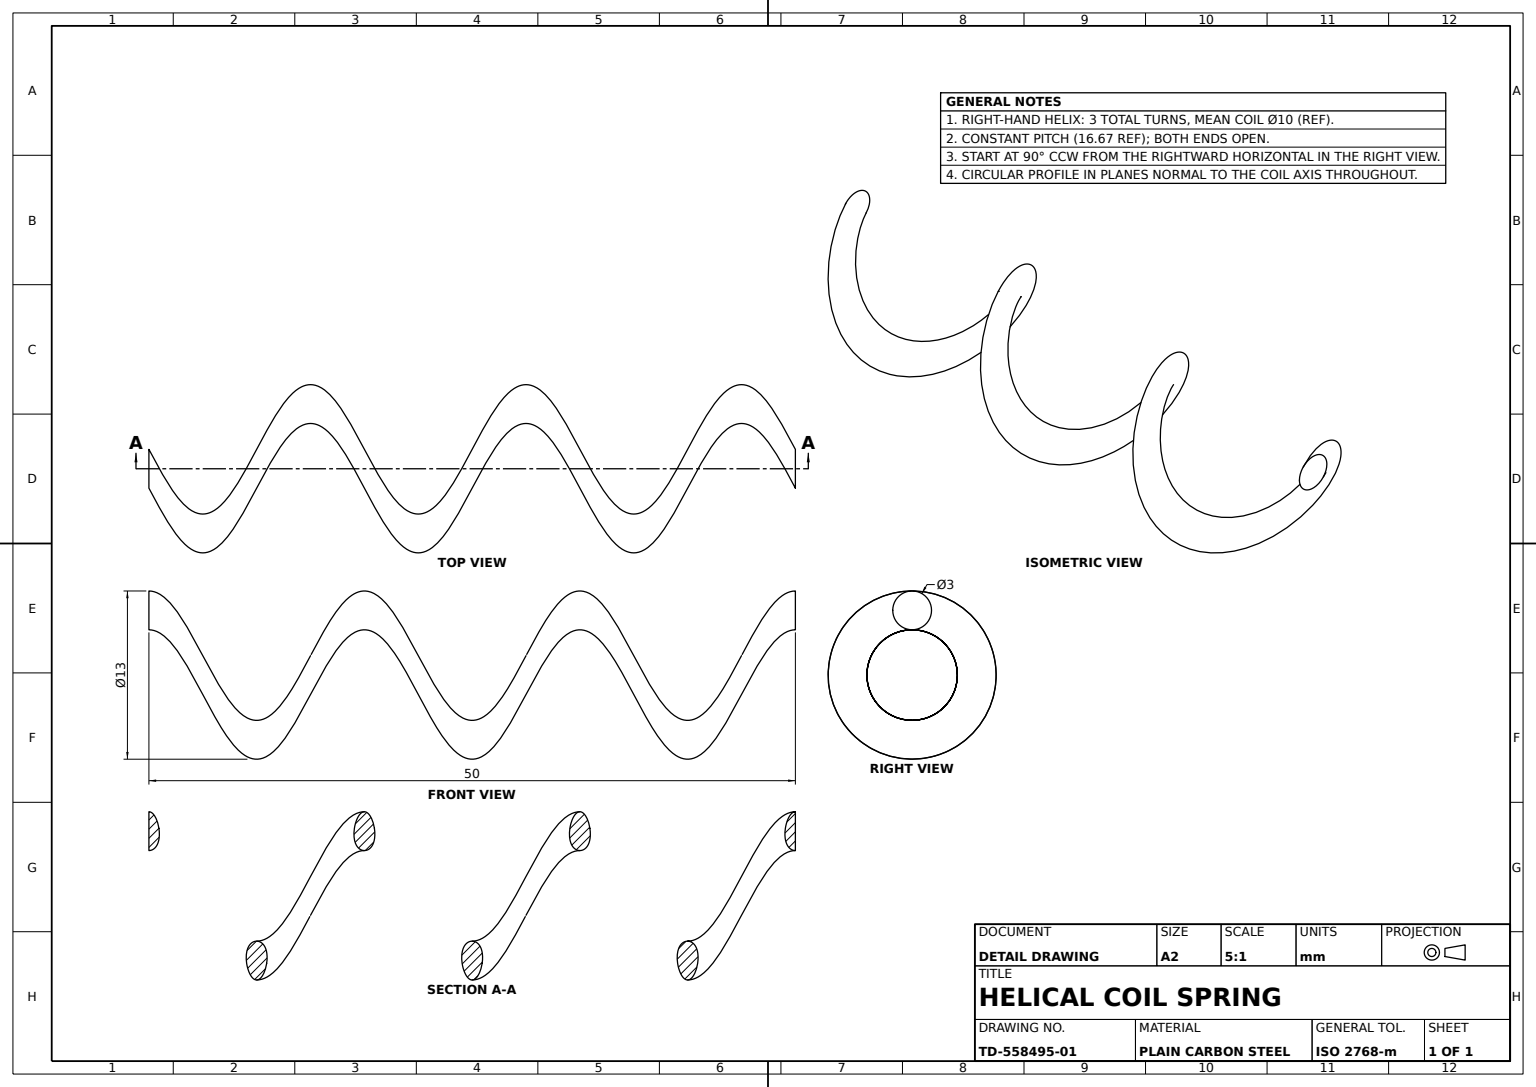
from build123d import *

# Parameters (mm, degrees)
SPRING_COIL_PITCH       = 16.666666667
SPRING_COIL_HEIGHT      = 50
SPRING_COIL_RADIUS      = 5
SPRING_COIL_START_ANGLE = 90
WIRE_PROFILE_R          = 1.5


with BuildPart() as part:
    # Spring Coil: sweep along a helix
    with BuildLine() as spring_coil_path:
        add(Helix(SPRING_COIL_PITCH, SPRING_COIL_HEIGHT, SPRING_COIL_RADIUS, center=(0, 0, 0), direction=(0, 0, 1), mode=Mode.PRIVATE).rotate(Axis((0, 0, 0), (0, 0, 1)), SPRING_COIL_START_ANGLE))
    # Wire Profile → Spring Coil (sweep)
    with BuildSketch(Plane.XY):
        with Locations((0, 5)):
            Circle(WIRE_PROFILE_R)
    sweep(path=spring_coil_path.line, is_frenet=True)


solid = part.part
